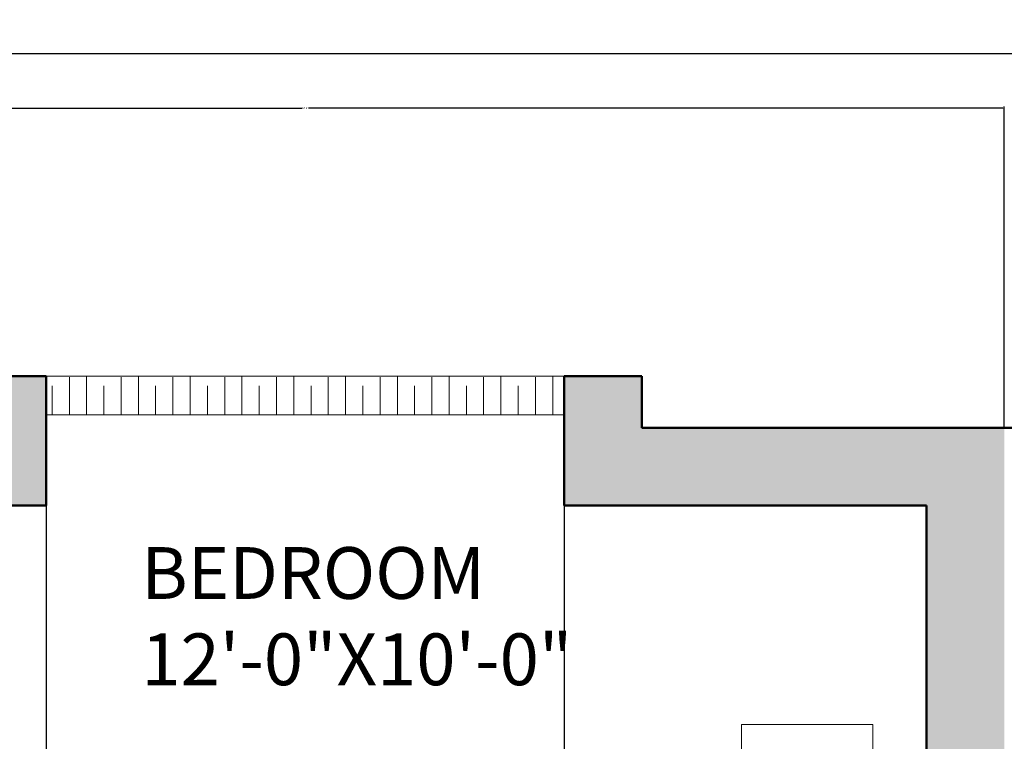
# Model space of a CAD drawing. Units: inches. Extents: x -12 to 604, y -566 to 58.
# Tile 7 of 12: x 166 to 280, y -25 to 58. Entities that reach past the tile are written whole.
import ezdxf

# ---------------------------------------------------------------- set-up
doc = ezdxf.new("R2010")
doc.units = ezdxf.units.IN
doc.header["$MEASUREMENT"] = 0
for name, color, linetype, lineweight in [('A-ANNO-DIMS', 2, 'Continuous', 18), ('A-AREA-IDEN', 7, 'Continuous', 18), ('A-FURN', 8, 'Continuous', 18), ('A-GLAZ', 82, 'Continuous', 18), ('A-GLAZ-PATT', 82, 'Continuous', 13), ('A-WALL', 7, 'Continuous', 50), ('A-WALL-PATT', 18, 'Continuous', 13)]:
    doc.layers.add(name, color=color, linetype=linetype, lineweight=lineweight)
doc.styles.get("Standard").update_dxf_attribs({"font": 'arial.ttf'})
doc.dimstyles.get("Standard").update_dxf_attribs({"dimtxt": 0.18, "dimasz": 0.18, "dimexe": 0.18, "dimexo": 0.0625, "dimgap": 0.09, "dimtad": 0, "dimtih": 1, "dimtoh": 1, "dimdec": 0, "dimzin": 0, "dimdsep": 46, "dimlunit": 3, "dimtxsty": 'Standard', "dimcen": 0.09, "dimadec": 0, "dimazin": 0, "dimtfac": 1, "dimtdec": 0, "dimtofl": 0, "dimtmove": 0, "dimatfit": 3, "dimfxl": 1, "dimtolj": 1, "dimtzin": 0, "dimarcsym": 0})

# ---------------------------------------------------------------- blocks, each defined once
blk = doc.blocks.new('*D4')
at = {"layer": 'A-ANNO-DIMS', "color": 0, "lineweight": -2, "transparency": 16777216}
for p, q in [((30.32, 11.2), (30.32, 54.68)), ((30.5, 54.5), (303.81, 54.5)), ((598.14, 54.5), (324.84, 54.5)), ((598.32, 11.2), (598.32, 54.68))]:
    blk.add_line(p, q, dxfattribs=at)
at = {"layer": 'A-ANNO-DIMS', "color": 0, "transparency": 16777216}
for points in [[(30.5, 54.53), (30.5, 54.47), (30.32, 54.5)], [(598.14, 54.53), (598.14, 54.47), (598.32, 54.5)]]:
    blk.add_solid(points, dxfattribs=at)
at = {"layer": 'Defpoints', "color": 0, "transparency": 16777216}
for p in [(598.32, 54.5), (30.32, 11.14), (598.32, 11.14)]:
    blk.add_point(p, dxfattribs=at)
at = {"layer": 'A-ANNO-DIMS', "color": 0, "transparency": 16777216, "insert": (314.32, 54.5), "char_height": 6, "attachment_point": 5}
blk.add_mtext('\\A1;47\'-4"', dxfattribs=at)
blk = doc.blocks.new('*D52')
at = {"layer": 'A-ANNO-DIMS', "color": 0, "lineweight": -2, "transparency": 16777216}
for p, q in [((118.32, 11.2), (118.32, 48.37)), ((118.5, 48.19), (198.93, 48.19)), ((280.14, 48.19), (199.71, 48.19)), ((280.32, 11.2), (280.32, 48.37))]:
    blk.add_line(p, q, dxfattribs=at)
at = {"layer": 'A-ANNO-DIMS', "color": 0, "transparency": 16777216}
for points in [[(118.5, 48.22), (118.5, 48.16), (118.32, 48.19)], [(280.14, 48.22), (280.14, 48.16), (280.32, 48.19)]]:
    blk.add_solid(points, dxfattribs=at)
at = {"layer": 'Defpoints', "color": 0, "transparency": 16777216}
for p in [(280.32, 48.19), (118.32, 11.14), (280.32, 11.14)]:
    blk.add_point(p, dxfattribs=at)
at = {"layer": 'A-ANNO-DIMS', "color": 0, "transparency": 16777216, "insert": (199.32, 48.19), "char_height": 0.18, "attachment_point": 5}
blk.add_mtext('\\A1;13\'-6"', dxfattribs=at)
blk = doc.blocks.new('*D57')
at = {"layer": 'A-ANNO-DIMS', "color": 0, "lineweight": -2, "transparency": 16777216}
for p, q in [((169.32, 12.58), (169.32, -565.59)), ((229.32, 12.58), (229.32, -565.59)), ((169.5, -565.41), (198.99, -565.41)), ((229.14, -565.41), (199.65, -565.41))]:
    blk.add_line(p, q, dxfattribs=at)
at = {"layer": 'A-ANNO-DIMS', "color": 0, "transparency": 16777216}
for points in [[(169.5, -565.38), (169.5, -565.44), (169.32, -565.41)], [(229.14, -565.38), (229.14, -565.44), (229.32, -565.41)]]:
    blk.add_solid(points, dxfattribs=at)
at = {"layer": 'Defpoints', "color": 0, "transparency": 16777216}
for p in [(169.32, 12.64), (229.32, 12.64), (229.32, -565.41)]:
    blk.add_point(p, dxfattribs=at)
at = {"layer": 'A-ANNO-DIMS', "color": 0, "transparency": 16777216, "insert": (199.32, -565.41), "char_height": 0.18, "attachment_point": 5}
blk.add_mtext('\\A1;5\'-0"', dxfattribs=at)

msp = doc.modelspace()

# ---------------------------------------------------------------- hatches: boundary and pattern name
at = {"layer": 'A-GLAZ-PATT'}
h = msp.add_hatch(dxfattribs=at)
h.set_pattern_fill('GOST_WOOD', color=256)
h.set_pattern_definition([(90, (0, 0), (6, -4e-16), [10, -2]), (90, (2, -2), (6, -4e-16), [6, -1.5, 3, -1.5]), (90, (4, -5), (6, -4e-16), [10, -2])])
h.paths.add_polyline_path([(229.32, 17.14), (169.32, 17.14), (169.32, 14.14), (169.32, 12.64), (229.32, 12.64)])
h.paths.add_polyline_path([(439.32, 17.14), (415.32, 17.14), (415.32, 12.64), (439.32, 12.64)])
h.paths.add_polyline_path([(472.32, 17.14), (448.32, 17.14), (448.32, 12.64), (472.32, 12.64)])
at = {"layer": 'A-WALL-PATT'}
h = msp.add_hatch(color=256, dxfattribs=at)
h.dxf.hatch_style = 1
h.paths.add_polyline_path([(169.32, 11.14), (169.32, 17.14), (160.32, 17.14), (160.32, 11.14), (118.32, 11.14), (118.32, 6.64), (118.32, 2.14), (127.32, 2.14), (169.32, 2.14)])
h.paths.add_polyline_path([(127.32, -13.61), (118.32, -13.61), (118.32, -29.36), (34.82, -29.36), (24.32, -29.36), (24.32, -38.36), (39.32, -38.36), (118.32, -38.36), (118.32, -126.86), (127.32, -126.86), (127.32, -117.86)])
h.paths.add_polyline_path([(82.32, -92.36), (39.32, -92.36), (39.32, -56.22), (30.32, -56.22), (24.32, -56.22), (24.32, -65.22), (30.32, -65.22), (30.32, -113.36), (24.32, -113.36), (24.32, -122.36), (39.32, -122.36), (39.32, -101.36), (82.32, -101.36), (82.32, -96.86)], flags=17)
h.paths.add_polyline_path([(280.32, 11.14), (238.32, 11.14), (238.32, 17.14), (229.32, 17.14), (229.32, 12.64), (229.32, 11.14), (229.32, 2.14), (271.32, 2.14), (271.32, -117.86), (163.32, -117.86), (163.32, -126.86), (271.32, -126.86), (271.32, -189.86), (280.32, -189.86), (280.32, -180.86)])
h.paths.add_polyline_path([(415.32, 17.14), (406.32, 17.14), (406.32, 11.14), (358.32, 11.14), (358.32, -21.86), (367.32, -21.86), (367.32, 2.14), (415.32, 2.14)], flags=17)
h.paths.add_polyline_path([(484.55, -45.86), (448.32, -45.86), (448.32, 2.14), (448.32, 17.14), (439.32, 17.14), (439.32, 12.64), (439.32, 2.14), (439.32, -45.86), (367.32, -45.86), (358.32, -45.86), (358.32, -54.86), (430.32, -54.86), (430.32, -69.59), (430.32, -180.86), (318.82, -180.86), (318.82, -189.86), (318.82, -331.86), (327.82, -331.86), (327.82, -189.86), (439.32, -189.86), (439.32, -180.86), (439.32, -54.86), (483.5, -54.86), (484.55, -54.86)])
h.paths.add_polyline_path([(529.32, 11.14), (481.32, 11.14), (481.32, 17.14), (472.32, 17.14), (472.32, 12.64), (472.32, 2.14), (520.32, 2.14), (520.32, -21.86), (529.32, -21.86)])
h.paths.add_polyline_path([(598.32, -45.86), (582.42, -45.86), (582.42, -50.36), (582.42, -54.86), (589.32, -54.86), (589.32, -99.86), (598.32, -99.86), (604.32, -99.86), (604.32, -90.86), (598.32, -90.86)])
h.paths.add_polyline_path([(598.32, -168.86), (604.32, -168.86), (604.32, -159.86), (589.32, -159.86), (589.32, -180.86), (477.32, -180.86), (477.32, -189.86), (477.32, -259.86), (486.32, -259.86), (486.32, -189.86), (589.32, -189.86), (589.32, -204.86), (598.32, -204.86), (604.32, -204.86), (604.32, -195.86), (598.32, -195.86)])
h.paths.add_polyline_path([(598.32, -244.86), (604.32, -244.86), (604.32, -235.86), (598.32, -235.86), (589.32, -235.86), (589.32, -250.86), (522.32, -250.86), (522.32, -259.86), (589.32, -259.86), (589.32, -274.86), (598.32, -274.86), (604.32, -274.86), (604.32, -265.86), (598.32, -265.86)])
h.paths.add_polyline_path([(598.32, -333.28), (604.32, -333.28), (604.32, -324.28), (598.32, -324.28), (598.32, -321.87), (598.32, -318.28), (604.32, -318.28), (604.32, -309.28), (598.32, -309.28), (589.32, -309.28), (589.32, -341.95), (589.38, -341.95), (589.38, -363.16), (589.32, -381.86), (565.32, -381.86), (565.32, -390.86), (589.32, -390.86), (589.32, -450.86), (598.32, -450.86), (604.32, -450.86), (604.32, -441.86), (598.32, -441.86), (598.32, -390.86), (604.32, -390.86), (604.32, -381.86), (598.32, -381.86)])
h.paths.add_polyline_path([(541.32, -345.86), (424.32, -345.86), (424.32, -354.86), (532.32, -354.86), (532.32, -474.86), (463.39, -474.86), (463.39, -483.86), (553.32, -483.86), (553.32, -474.86), (541.32, -474.86), (541.32, -390.86), (541.32, -381.86)])
h.paths.add_polyline_path([(604.32, -474.86), (589.32, -474.86), (553.32, -474.86), (553.32, -483.86), (598.32, -483.86), (604.32, -483.86)])
h.paths.add_polyline_path([(388.32, -483.86), (388.32, -474.86), (388.32, -460.13), (388.32, -333.86), (388.32, -322.86), (379.32, -322.86), (379.32, -331.86), (379.32, -333.86), (379.32, -474.86), (379.32, -520.86), (344.32, -520.86), (344.32, -529.86), (379.32, -529.86), (388.32, -529.86)])
h.paths.add_polyline_path([(284.32, -520.86), (249.32, -520.86), (249.32, -474.86), (249.32, -368.36), (240.32, -368.36), (240.32, -474.86), (238.52, -474.86), (238.52, -483.86), (240.32, -483.86), (240.32, -529.86), (249.32, -529.86), (284.32, -529.86)])
h.paths.add_polyline_path([(178.82, -474.86), (158.91, -474.86), (158.91, -483.86), (162.32, -483.86), (178.82, -483.86)])
h.paths.add_polyline_path([(84.32, -474.86), (84.32, -366.86), (75.32, -366.86), (75.32, -474.86), (39.32, -474.86), (39.32, -453.86), (24.32, -453.86), (24.32, -462.86), (30.32, -462.86), (30.32, -483.86), (84.32, -483.86)])
h.paths.add_polyline_path([(39.32, -342.86), (75.32, -342.86), (84.32, -342.86), (179.67, -342.86), (179.67, -333.86), (39.32, -333.86), (39.32, -318.86), (24.32, -318.86), (24.32, -327.86), (30.32, -327.86), (30.32, -432.86), (24.32, -432.86), (24.32, -441.86), (30.32, -441.86), (39.32, -441.86)])
h.paths.add_polyline_path([(249.32, -252.86), (115.32, -252.86), (115.32, -225.86), (106.32, -225.86), (106.32, -252.86), (39.32, -252.86), (39.32, -237.86), (24.32, -237.86), (24.32, -246.86), (30.32, -246.86), (30.32, -267.86), (24.32, -267.86), (24.32, -276.86), (39.32, -276.86), (39.32, -261.86), (240.32, -261.86), (240.32, -331.86), (249.32, -331.86), (266.82, -331.86), (266.82, -322.86), (249.32, -322.86)])
h.paths.add_polyline_path([(127.32, -180.86), (39.32, -180.86), (24.32, -180.86), (24.32, -189.86), (39.32, -189.86), (127.32, -189.86)])
h.paths.add_polyline_path([(39.32, -159.86), (24.32, -159.86), (24.32, -168.86), (30.32, -168.86), (30.32, -180.86), (39.32, -180.86)])
h.paths.add_polyline_path([(470.51, -17.27), (512.48, -17.27), (512.48, 5.12), (470.51, 5.12)], flags=9)
h.paths.add_polyline_path([(484.21, -244.26), (526.45, -244.26), (526.45, -221.87), (484.21, -221.87)], flags=24)
h.paths.add_polyline_path([(36.91, -442.88), (83.54, -442.88), (83.54, -420.5), (36.91, -420.5)], flags=25)

# ---------------------------------------------------------------- linework, layer by layer
at = {"layer": 'A-FURN'}
msp.add_line((265.09, -23.23), (265.09, -114.65), dxfattribs=at)
msp.add_lwpolyline([(249.86, -41.51), (249.86, -23.23), (265.09, -23.23)], dxfattribs=at)
at = {"layer": 'A-GLAZ'}
for p, q in [((169.32, 17.14), (229.32, 17.14)), ((169.32, 12.64), (169.32, 17.14)), ((169.32, 17.14), (169.32, 14.14)), ((229.32, 17.14), (229.32, 12.64)), ((229.32, 12.64), (169.32, 12.64))]:
    msp.add_line(p, q, dxfattribs=at)
at = {"layer": 'A-WALL'}
for p, q in [((160.32, 17.14), (169.32, 17.14)), ((169.32, 11.14), (169.32, 17.14)), ((229.32, 17.14), (229.32, 11.14)), ((229.32, 17.14), (238.32, 17.14)), ((238.32, 17.14), (238.32, 11.14)), ((169.32, 2.14), (169.32, 11.14)), ((229.32, 11.14), (229.32, 2.14)), ((238.32, 11.14), (406.32, 11.14)), ((127.32, 2.14), (169.32, 2.14)), ((229.32, 2.14), (271.32, 2.14)), ((271.32, 2.14), (271.32, -117.86))]:
    msp.add_line(p, q, dxfattribs=at)

# ---------------------------------------------------------------- texts
at = {"layer": 'A-AREA-IDEN', "insert": (180.34, -2.68), "char_height": 6, "attachment_point": 1}
msp.add_mtext('BEDROOM\\P12\'-0"X10\'-0"', dxfattribs=at)

# ---------------------------------------------------------------- dimensions: what is measured, and where the dimension line sits
at = {"layer": 'A-ANNO-DIMS'}
for base, p1, p2, override, picture, middle in [((598.32, 54.5), (30.32, 11.14), (598.32, 11.14), {"dimtxt": 6, "dimclrd": 0, "dimclre": 0, "dimclrt": 0}, '*D4', (314.32, 54.5)), ((280.32, 48.19), (118.32, 11.14), (280.32, 11.14), {"dimdec": 1, "dimlfac": 1, "dimrnd": 0, "dimzin": 1, "dimdsep": 46, "dimlunit": 4, "dimfrac": 2}, '*D52', (199.32, 48.19)), ((229.32, -565.41), (169.32, 12.64), (229.32, 12.64), {"dimdec": 1, "dimlfac": 1, "dimrnd": 0, "dimzin": 1, "dimdsep": 46, "dimlunit": 4, "dimfrac": 2}, '*D57', (199.32, -565.41))]:
    dim = msp.add_linear_dim(base=base, p1=p1, p2=p2, dimstyle='Standard', override=override, dxfattribs=at)
    dim.commit()
    dim.dimension.update_dxf_attribs({"geometry": picture, "text_midpoint": middle})

doc.saveas('drawing.dxf')
